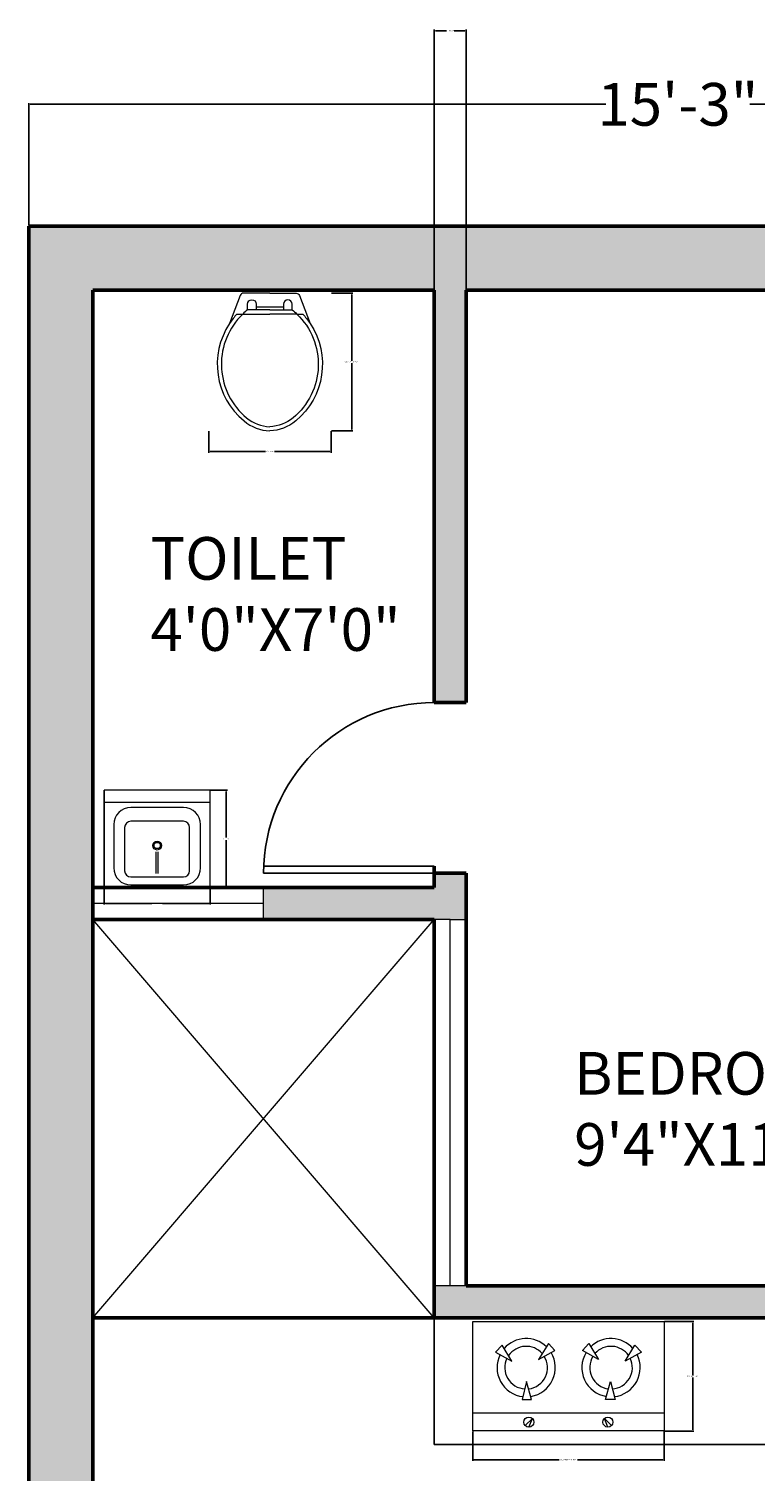
# Model space of a CAD drawing. Units: inches. Extents: x 3 to 485, y -522 to 42.
# Tile 3 of 6: x 30 to 132, y -161 to 42. Entities that reach past the tile are written whole.
import ezdxf

# ---------------------------------------------------------------- set-up
doc = ezdxf.new("R2010")
doc.units = ezdxf.units.IN
doc.header["$MEASUREMENT"] = 0
for name, color, linetype, lineweight in [('A-ANNO-DIMS', 2, 'Continuous', 18), ('A-AREA-IDEN', 7, 'Continuous', 18), ('A-DOOR', 3, 'Continuous', 25), ('A-EQPM', 8, 'Continuous', 18), ('A-FLOR-CASE', 8, 'Continuous', 25), ('A-FLOR-FIXT', 9, 'Continuous', 18), ('A-FLOR-OPEN', 8, 'Continuous', 18), ('A-GLAZ', 4, 'Continuous', 18), ('A-WALL', 7, 'Continuous', 50)]:
    doc.layers.add(name, color=color, linetype=linetype, lineweight=lineweight)
doc.layers.add('A-WALL-PATT', color=18, linetype='Continuous', lineweight=13, true_color=0x000000)
doc.styles.get("Standard").update_dxf_attribs({"font": 'arial.ttf'})
doc.dimstyles.get("Standard").update_dxf_attribs({"dimtxt": 0.18, "dimasz": 0.18, "dimexe": 0.18, "dimexo": 0.0625, "dimgap": 0.09, "dimtad": 0, "dimtih": 1, "dimtoh": 1, "dimdec": 0, "dimzin": 0, "dimdsep": 46, "dimlunit": 3, "dimtxsty": 'Standard', "dimcen": 0.09, "dimadec": 0, "dimazin": 0, "dimtfac": 1, "dimtdec": 0, "dimtofl": 0, "dimtmove": 0, "dimatfit": 3, "dimfxl": 1, "dimtolj": 1, "dimtzin": 0, "dimarcsym": 0})

# ---------------------------------------------------------------- blocks, each defined once
blk = doc.blocks.new('М14 600х655')
for p, q in [((-655, 600), (-655, 0)), ((-655, 600), (-655, 0)), ((-655, 0), (-655, 600)), ((0, 600), (-655, 600)), ((0, 0), (0, 600)), ((0, 525), (-655, 525)), ((-165.1, 494.1), (-489.9, 494.1)), ((-595.8, 388.1), (-595.8, 121.3)), ((-528.4, 370.1), (-528.4, 103.3)), ((-165.4, 408.4), (-490.2, 408.4)), ((-127.2, 103.3), (-127.2, 370.1)), ((-59.2, 121.3), (-59.2, 388.1)), ((-333.5, 87.1), (-333.5, 219.6)), ((-321.5, 87.1), (-321.5, 219.6)), ((-655, 0), (-655, 0)), ((-655, 0), (-655, 0)), ((-655, 0), (0, 0)), ((-655, 0), (0, 0)), ((-490.2, 65.1), (-165.4, 65.1)), ((-489.9, 15.4), (-165.1, 15.4))]:
    blk.add_line(p, q)
for radius in [27.6, 19.3]:
    blk.add_circle((-327.5, 258.9), radius)
for centre, radius, start, end in [((-489.9, 388.1), 105.9, 90, 180), ((-165.1, 388.1), 105.9, 0, 90), ((-490.2, 370.1), 38.2, 90, 180), ((-165.4, 370.1), 38.2, 0, 90), ((-489.9, 121.3), 105.9, 180, 270), ((-490.2, 103.3), 38.2, 180, 270), ((-165.4, 103.3), 38.2, 270, 0), ((-165.1, 121.3), 105.9, 270, 0)]:
    blk.add_arc(centre, radius, start, end)
blk = doc.blocks.new('*D4')
at = {"layer": 'A-ANNO-DIMS', "color": 0, "lineweight": -2, "transparency": 16777216}
for p, q in [((30.29, 14.07), (30.29, 31.29)), ((30.47, 31.11), (111.43, 31.11)), ((212.61, 31.11), (131.65, 31.11)), ((212.79, 14.07), (212.79, 31.29))]:
    blk.add_line(p, q, dxfattribs=at)
at = {"layer": 'A-ANNO-DIMS', "color": 0, "transparency": 16777216}
for points in [[(30.47, 31.14), (30.47, 31.08), (30.29, 31.11)], [(212.61, 31.14), (212.61, 31.08), (212.79, 31.11)]]:
    blk.add_solid(points, dxfattribs=at)
at = {"layer": 'Defpoints', "color": 0, "transparency": 16777216}
for p in [(212.79, 31.11), (30.29, 14), (212.79, 14)]:
    blk.add_point(p, dxfattribs=at)
at = {"layer": 'A-ANNO-DIMS', "color": 0, "transparency": 16777216, "insert": (121.54, 31.11), "char_height": 6, "attachment_point": 5}
blk.add_mtext('\\A1;15\'-3"', dxfattribs=at)
blk = doc.blocks.new('WC-PLAN')
for p, q in [((2.77, 16.42), (3.59, 16.42)), ((3.59, 16.42), (7.39, 16.42)), ((11.2, 16.42), (7.39, 16.42)), ((11.2, 16.42), (12.01, 16.42))]:
    blk.add_line(p, q)
for points in [[(7.39, 19.36), (3.7, 19.36, 0.31031), (3.24, 19.04), (1.73, 15.1, 0.209071)], [(4.25, 17.01), (4.25, 17.82, -1), (5.49, 17.82), (5.49, 17.4)], [(7.39, 19.36), (11.09, 19.36, -0.31031), (11.54, 19.04), (13.06, 15.1, -0.209071)], [(10.53, 17.01), (10.53, 17.82, 1), (9.3, 17.82), (9.3, 17.4)], [(2.77, 16.42, 0.040937), (1.73, 15.1, 0.163732)], [(3.59, 16.42, 0.014165), (3.2, 16.03, 0.162618)], [(4.25, 17.01, 0.022712), (3.59, 16.42, 0.162618)], [(7.39, 17.01), (4.25, 17.01, 0.022712)], [(7.39, 17.01), (10.53, 17.01, -0.476108)], [(11.2, 16.42, -0.448546), (10.66, 1.84, -0.162618), (7.39, 0.58, -0.470877)], [(10.53, 17.01, -0.022712), (11.2, 16.42, -0.162618)], [(12.01, 16.42, -0.040937), (13.06, 15.1, -0.163732)], [(1.73, 15.1, 0.383919), (3.76, 1.39, 0.163732), (7.39, 0, 0.359733)], [(3.2, 16.03, 0.431639), (4.12, 1.84, 0.162618), (7.39, 0.58, 0.470877)], [(13.06, 15.1, -0.383919), (11.03, 1.39, -0.163732), (7.39, 0, -0.359733)]]:
    blk.add_lwpolyline(points, format="xyb")
for points in [[(9.3, 17.4), (5.49, 17.4)], [(5.49, 17.4), (5.49, 17.01)], [(9.3, 17.4), (9.3, 17.01)]]:
    blk.add_lwpolyline(points)
blk = doc.blocks.new('COOKTOP-TWO-BURNER')
for p, q in [((10.65, 12.28), (9.27, 10.05)), ((11.55, 11.31), (10.65, 12.28)), ((15.42, 11.31), (16.32, 12.28)), ((16.32, 12.28), (17.71, 10.05)), ((4.16, 12.04), (3.23, 11.09)), ((3.23, 11.09), (5.52, 9.82)), ((5.52, 9.82), (4.16, 12.04)), ((9.27, 10.05), (11.55, 11.31)), ((17.71, 10.05), (15.42, 11.31)), ((21.45, 9.82), (22.81, 12.04)), ((23.74, 11.09), (21.45, 9.82)), ((22.81, 12.04), (23.74, 11.09)), ((7.59, 6.96), (6.96, 4.43)), ((8.29, 4.43), (7.59, 6.96)), ((18.68, 4.43), (19.38, 6.96)), ((19.38, 6.96), (20.01, 4.43)), ((6.96, 4.43), (8.29, 4.43)), ((20.01, 4.43), (18.68, 4.43)), ((26.9, 2.5), (0, 2.5))]:
    blk.add_line(p, q)
at = {"ltscale": 20}
for p, q in [((8.39, 1.74), (7.39, 0.75)), ((7.89, 0.54), (8.39, 1.74)), ((18.51, 1.74), (19.51, 0.75)), ((19.01, 0.54), (18.51, 1.74))]:
    blk.add_line(p, q, dxfattribs=at)
blk.add_lwpolyline([(0, 15.37), (26.9, 15.37), (26.9, 0), (0, 0)], close=True)
for centre in [(7.89, 1.25), (19.01, 1.25)]:
    blk.add_circle(centre, 0.707, dxfattribs=at)
for centre, radius, start, end in [((7.52, 8.9), 4.1, 45.8373, 138.7775), ((19.45, 8.9), 4.1, 41.2225, 134.1627), ((7.52, 8.9), 4.1, 153.231, 263.5995), ((7.52, 8.9), 3, 154.0793, 266.4247), ((7.52, 8.9), 3, 41.1973, 145.4439), ((7.52, 8.9), 3, 276.98, 32.0222), ((7.52, 8.9), 4.1, 279.2438, 31.147), ((19.45, 8.9), 4.1, 148.853, 260.7562), ((19.45, 8.9), 3, 147.9778, 263.02), ((19.45, 8.9), 3, 34.5561, 138.8027), ((19.45, 8.9), 3, 273.5753, 25.9207), ((19.45, 8.9), 4.1, 276.4005, 26.769)]:
    blk.add_arc(centre, radius, start, end)
blk = doc.blocks.new('DOOR-SWING-24IN')
for p, q in [((-1, 0), (-1, 24)), ((0, 0), (0, 24))]:
    blk.add_line(p, q)
blk.add_arc((0, 0), 24, 90, 180)
blk = doc.blocks.new('*D22')
at = {"layer": 'A-ANNO-DIMS', "color": 0, "lineweight": -2, "transparency": 16777216}
for p, q in [((72.84, 4.56), (75.86, 4.56)), ((75.68, 4.38), (75.68, -4.94)), ((75.68, -14.62), (75.68, -5.3)), ((72.84, -14.8), (75.86, -14.8))]:
    blk.add_line(p, q, dxfattribs=at)
at = {"layer": 'A-ANNO-DIMS', "color": 0, "transparency": 16777216}
for points in [[(75.65, 4.38), (75.71, 4.38), (75.68, 4.56)], [(75.65, -14.62), (75.71, -14.62), (75.68, -14.8)]]:
    blk.add_solid(points, dxfattribs=at)
at = {"layer": 'Defpoints', "color": 0, "transparency": 16777216}
for p in [(72.78, 4.56), (75.68, 4.56), (72.78, -14.8)]:
    blk.add_point(p, dxfattribs=at)
at = {"layer": 'A-ANNO-DIMS', "color": 0, "transparency": 16777216, "insert": (75.68, -5.12), "char_height": 0.18, "attachment_point": 5}
blk.add_mtext('\\A1;WC 1\'-7 1/2" TYP.', dxfattribs=at)
blk = doc.blocks.new('*D23')
at = {"layer": 'A-ANNO-DIMS', "color": 0, "lineweight": -2, "transparency": 16777216}
for p, q in [((55.58, -14.86), (55.58, -17.88)), ((72.78, -14.86), (72.78, -17.88)), ((55.76, -17.7), (63.55, -17.7)), ((72.6, -17.7), (64.81, -17.7))]:
    blk.add_line(p, q, dxfattribs=at)
at = {"layer": 'A-ANNO-DIMS', "color": 0, "transparency": 16777216}
for points in [[(55.76, -17.67), (55.76, -17.73), (55.58, -17.7)], [(72.6, -17.67), (72.6, -17.73), (72.78, -17.7)]]:
    blk.add_solid(points, dxfattribs=at)
at = {"layer": 'Defpoints', "color": 0, "transparency": 16777216}
for p in [(55.58, -14.8), (72.78, -14.8), (72.78, -17.7)]:
    blk.add_point(p, dxfattribs=at)
at = {"layer": 'A-ANNO-DIMS', "color": 0, "transparency": 16777216, "insert": (64.18, -17.7), "char_height": 0.18, "attachment_point": 5}
blk.add_mtext('\\A1;1\'-5" TYP.', dxfattribs=at)
blk = doc.blocks.new('*D24')
at = {"layer": 'A-ANNO-DIMS', "color": 0, "lineweight": -2, "transparency": 16777216}
for p, q in [((92.69, -155.48), (92.69, -159.63)), ((119.59, -155.48), (119.59, -159.63)), ((92.87, -159.45), (104.84, -159.45)), ((119.41, -159.45), (107.44, -159.45))]:
    blk.add_line(p, q, dxfattribs=at)
at = {"layer": 'A-ANNO-DIMS', "color": 0, "transparency": 16777216}
for points in [[(92.87, -159.42), (92.87, -159.48), (92.69, -159.45)], [(119.41, -159.42), (119.41, -159.48), (119.59, -159.45)]]:
    blk.add_solid(points, dxfattribs=at)
at = {"layer": 'Defpoints', "color": 0, "transparency": 16777216}
for p in [(92.69, -155.42), (119.59, -155.42), (119.59, -159.45)]:
    blk.add_point(p, dxfattribs=at)
at = {"layer": 'A-ANNO-DIMS', "color": 0, "transparency": 16777216, "insert": (106.14, -159.45), "char_height": 0.18, "attachment_point": 5}
blk.add_mtext('\\A1;COOKTOP 2\'-3" TYP.', dxfattribs=at)
blk = doc.blocks.new('*D25')
at = {"layer": 'A-ANNO-DIMS', "color": 0, "lineweight": -2, "transparency": 16777216}
for p, q in [((119.65, -140.04), (123.8, -140.04)), ((123.62, -140.22), (123.62, -147.55)), ((123.62, -155.24), (123.62, -147.91)), ((119.65, -155.42), (123.8, -155.42))]:
    blk.add_line(p, q, dxfattribs=at)
at = {"layer": 'A-ANNO-DIMS', "color": 0, "transparency": 16777216}
for points in [[(123.59, -140.22), (123.65, -140.22), (123.62, -140.04)], [(123.59, -155.24), (123.65, -155.24), (123.62, -155.42)]]:
    blk.add_solid(points, dxfattribs=at)
at = {"layer": 'Defpoints', "color": 0, "transparency": 16777216}
for p in [(119.59, -140.04), (123.62, -140.04), (119.59, -155.42)]:
    blk.add_point(p, dxfattribs=at)
at = {"layer": 'A-ANNO-DIMS', "color": 0, "transparency": 16777216, "insert": (123.62, -147.73), "char_height": 0.18, "attachment_point": 5}
blk.add_mtext('\\A1;1\'-3 1/2" TYP.', dxfattribs=at)
blk = doc.blocks.new('*D30')
at = {"layer": 'A-ANNO-DIMS', "color": 0, "lineweight": -2, "transparency": 16777216}
for p, q in [((40.87, -79.06), (40.87, -81.41)), ((55.79, -79.06), (55.79, -81.41)), ((41.05, -81.23), (47.59, -81.23)), ((55.61, -81.23), (49.06, -81.23))]:
    blk.add_line(p, q, dxfattribs=at)
at = {"layer": 'A-ANNO-DIMS', "color": 0, "transparency": 16777216}
for points in [[(41.05, -81.2), (41.05, -81.26), (40.87, -81.23)], [(55.61, -81.2), (55.61, -81.26), (55.79, -81.23)]]:
    blk.add_solid(points, dxfattribs=at)
at = {"layer": 'Defpoints', "color": 0, "transparency": 16777216}
for p in [(40.87, -79), (55.79, -79), (55.79, -81.23)]:
    blk.add_point(p, dxfattribs=at)
at = {"layer": 'A-ANNO-DIMS', "color": 0, "transparency": 16777216, "insert": (48.33, -81.23), "char_height": 0.18, "attachment_point": 5}
blk.add_mtext('\\A1;BASIN 1\'-3"', dxfattribs=at)
blk = doc.blocks.new('*D31')
at = {"layer": 'A-ANNO-DIMS', "color": 0, "lineweight": -2, "transparency": 16777216}
for p, q in [((55.85, -65.33), (58.21, -65.33)), ((58.03, -65.51), (58.03, -71.98)), ((58.03, -78.82), (58.03, -72.35)), ((55.85, -79), (58.21, -79))]:
    blk.add_line(p, q, dxfattribs=at)
at = {"layer": 'A-ANNO-DIMS', "color": 0, "transparency": 16777216}
for points in [[(58, -65.51), (58.06, -65.51), (58.03, -65.33)], [(58, -78.82), (58.06, -78.82), (58.03, -79)]]:
    blk.add_solid(points, dxfattribs=at)
at = {"layer": 'Defpoints', "color": 0, "transparency": 16777216}
for p in [(55.79, -65.33), (58.03, -65.33), (55.79, -79)]:
    blk.add_point(p, dxfattribs=at)
at = {"layer": 'A-ANNO-DIMS', "color": 0, "transparency": 16777216, "insert": (58.03, -72.16), "char_height": 0.18, "attachment_point": 5}
blk.add_mtext('\\A1;1\'-1 1/2"', dxfattribs=at)
blk = doc.blocks.new('*D36')
at = {"layer": 'A-ANNO-DIMS', "color": 0, "lineweight": -2, "transparency": 16777216}
for p, q in [((87.29, -52.93), (87.29, 41.63)), ((87.47, 41.45), (89, 41.45)), ((91.61, 41.45), (90.08, 41.45)), ((91.79, -52.93), (91.79, 41.63))]:
    blk.add_line(p, q, dxfattribs=at)
at = {"layer": 'A-ANNO-DIMS', "color": 0, "transparency": 16777216}
for points in [[(87.47, 41.48), (87.47, 41.42), (87.29, 41.45)], [(91.61, 41.48), (91.61, 41.42), (91.79, 41.45)]]:
    blk.add_solid(points, dxfattribs=at)
at = {"layer": 'Defpoints', "color": 0, "transparency": 16777216}
for p in [(91.79, 41.45), (87.29, -53), (91.79, -53)]:
    blk.add_point(p, dxfattribs=at)
at = {"layer": 'A-ANNO-DIMS', "color": 0, "transparency": 16777216, "insert": (89.54, 41.45), "char_height": 0.18, "attachment_point": 5}
blk.add_mtext('\\A1;0\'-4 1/2"', dxfattribs=at)

msp = doc.modelspace()

# ---------------------------------------------------------------- hatches: boundary and pattern name
at = {"layer": 'A-WALL-PATT'}
h = msp.add_hatch(color=256, dxfattribs=at)
h.dxf.hatch_style = 1
h.paths.add_polyline_path([(177.79, -240), (177.79, -235.5), (39.29, -235.5), (39.29, 5), (87.29, 5), (87.29, -53), (91.79, -53), (91.79, 5), (203.79, 5), (203.79, -477.5), (212.79, -477.5), (212.79, 14), (30.29, 14), (30.29, -477.5), (39.29, -477.5), (39.29, -388.5), (94.55, -388.5), (94.55, -384), (39.29, -384), (39.29, -240)])
h.paths.add_polyline_path([(142.75, -477.5), (142.75, -468.5), (82.75, -468.5), (82.75, -477.5)], flags=17)
h.paths.add_polyline_path([(63.29, -79), (63.29, -83.5), (87.29, -83.5), (89.54, -83.5), (91.79, -83.5), (91.79, -77), (87.29, -77), (87.29, -79)], flags=17)
h.paths.add_polyline_path([(177.79, -139.5), (177.79, -135), (91.79, -135), (87.29, -135), (87.29, -139.5), (91.79, -139.5)], flags=17)

# ---------------------------------------------------------------- linework, layer by layer
at = {"layer": 'A-FLOR-CASE'}
for p, q in [((87.29, -139.5), (87.29, -157.31)), ((87.29, -157.31), (177.79, -157.31))]:
    msp.add_line(p, q, dxfattribs=at)
at = {"layer": 'A-FLOR-OPEN'}
for p, q in [((39.29, -139.5), (87.29, -83.5)), ((87.29, -139.5), (39.29, -83.5))]:
    msp.add_line(p, q, dxfattribs=at)
at = {"layer": 'A-GLAZ'}
for p, q in [((63.29, -83.5), (63.29, -79)), ((63.29, -79), (63.29, -79)), ((63.29, -81.25), (39.29, -81.25)), ((89.54, -83.5), (87.29, -83.5)), ((89.54, -135), (89.54, -83.5)), ((89.54, -83.5), (91.79, -83.5)), ((91.79, -135), (87.29, -135))]:
    msp.add_line(p, q, dxfattribs=at)
at = {"layer": 'A-WALL'}
for p, q in [((30.29, 14), (30.29, -477.5)), ((30.29, 14), (212.79, 14)), ((39.29, 5), (87.29, 5)), ((39.29, 5), (39.29, -235.5)), ((87.29, 5), (87.29, -53)), ((91.79, 5), (91.79, -53)), ((91.79, 5), (203.79, 5)), ((87.29, -53), (91.79, -53)), ((87.29, -76), (87.29, -79)), ((87.29, -77), (91.79, -77)), ((91.79, -77), (91.79, -135)), ((39.29, -79), (87.29, -79)), ((39.29, -83.5), (87.29, -83.5)), ((87.29, -83.5), (87.29, -139.5)), ((91.79, -135), (177.79, -135)), ((91.79, -139.5), (39.29, -139.5)), ((91.79, -139.5), (177.79, -139.5))]:
    msp.add_line(p, q, dxfattribs=at)

# ---------------------------------------------------------------- block references
at = {"layer": 'A-DOOR', "extrusion": (0, 0, -1), "zscale": -1, "rotation": 269.9999999999999}
msp.add_blockref('DOOR-SWING-24IN', (-87.29, -77), dxfattribs=at)
at = {"layer": 'A-EQPM'}
msp.add_blockref('COOKTOP-TWO-BURNER', (92.69, -155.41), dxfattribs=at)
at = {"layer": 'A-FLOR-FIXT'}
msp.add_blockref('WC-PLAN', (56.78, -14.8), dxfattribs=at)
at = {"layer": 'A-FLOR-FIXT', "xscale": 0.0227811130337516, "yscale": 0.0227811130337516, "zscale": 0.0227811130337516}
msp.add_blockref('М14 600х655', (55.79, -79), dxfattribs=at)

# ---------------------------------------------------------------- texts
at = {"layer": 'A-AREA-IDEN', "char_height": 6, "attachment_point": 1}
for s, insert in [('TOILET\\P4\'0"X7\'0"', (47.38, -29.73)), ('BEDROOM\\P9\'4"X11\'8"', (106.96, -102.13))]:
    msp.add_mtext(s, dxfattribs=dict(at, insert=insert))

# ---------------------------------------------------------------- dimensions: what is measured, and where the dimension line sits
at = {"layer": 'A-ANNO-DIMS'}
for base, p1, p2, override, picture, middle in [((91.79, 41.45), (87.29, -53), (91.79, -53), {"dimdec": 1, "dimlfac": 1, "dimrnd": 0, "dimzin": 1, "dimdsep": 46, "dimlunit": 4, "dimfrac": 2}, '*D36', (89.54, 41.45)), ((212.79082571, 31.10517539), (30.29082571, 14.00352841), (212.79082571, 14.00352841), {"dimtxt": 6, "dimclrd": 0, "dimclre": 0, "dimclrt": 0}, '*D4', (121.54082571, 31.10517539))]:
    dim = msp.add_linear_dim(base=base, p1=p1, p2=p2, dimstyle='Standard', override=override, dxfattribs=at)
    dim.commit()
    dim.dimension.update_dxf_attribs({"geometry": picture, "text_midpoint": middle})
for base, p1, p2, text, picture, middle in [((75.68, 4.56), (72.78, -14.8), (72.78, 4.56), 'WC <> TYP.', '*D22', (75.68, -5.12)), ((123.62, -140.04), (119.59, -155.42), (119.59, -140.04), '<> TYP.', '*D25', (123.62, -147.73))]:
    dim = msp.add_linear_dim(base=base, p1=p1, p2=p2, angle=90, text=text, dimstyle='Standard', override={"dimdec": 1, "dimlfac": 1, "dimrnd": 0, "dimzin": 1, "dimdsep": 46, "dimlunit": 4, "dimfrac": 2}, dxfattribs=at)
    dim.commit()
    dim.dimension.update_dxf_attribs({"geometry": picture, "text_midpoint": middle})
for base, p1, p2, text, picture, middle in [((72.78, -17.7), (55.58, -14.8), (72.78, -14.8), '<> TYP.', '*D23', (64.18, -17.7)), ((55.79, -81.23), (40.87, -79), (55.79, -79), 'BASIN <>', '*D30', (48.33, -81.23)), ((119.59, -159.45), (92.69, -155.42), (119.59, -155.42), 'COOKTOP <> TYP.', '*D24', (106.14, -159.45))]:
    dim = msp.add_linear_dim(base=base, p1=p1, p2=p2, text=text, dimstyle='Standard', override={"dimdec": 1, "dimlfac": 1, "dimrnd": 0, "dimzin": 1, "dimdsep": 46, "dimlunit": 4, "dimfrac": 2}, dxfattribs=at)
    dim.commit()
    dim.dimension.update_dxf_attribs({"geometry": picture, "text_midpoint": middle})
dim = msp.add_linear_dim(base=(58.03, -65.33), p1=(55.79, -79), p2=(55.79, -65.33), angle=90, dimstyle='Standard', override={"dimdec": 1, "dimlfac": 1, "dimrnd": 0, "dimzin": 1, "dimdsep": 46, "dimlunit": 4, "dimfrac": 2}, dxfattribs=at)
dim.commit()
dim.dimension.update_dxf_attribs({"geometry": '*D31', "text_midpoint": (58.03, -72.16)})

doc.saveas('drawing.dxf')
